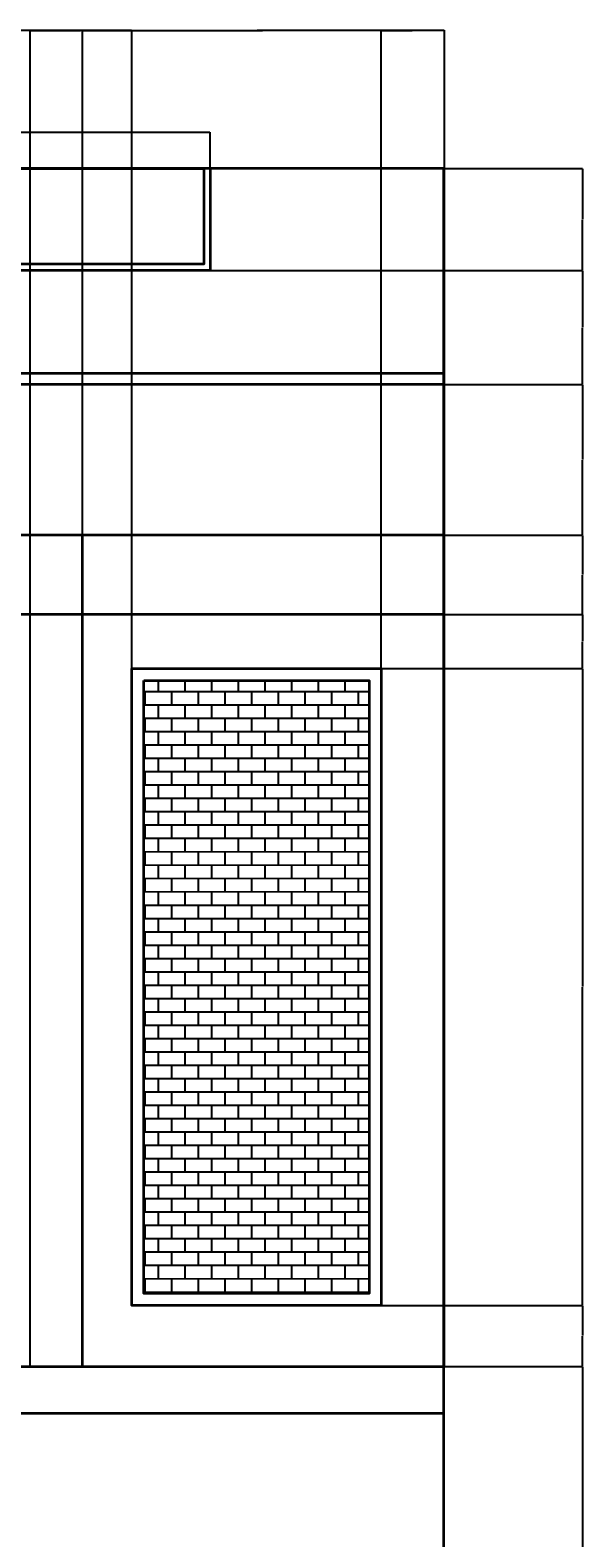
# Model space of a CAD drawing. Units: inches. Extents: x 1231 to 2151, y 481 to 2277.
# Tile 7 of 7: x 1819 to 2151, y 1373 to 2277. Entities that reach past the tile are written whole.
import ezdxf

# ---------------------------------------------------------------- set-up
doc = ezdxf.new("R2010")
doc.units = ezdxf.units.IN
doc.header["$MEASUREMENT"] = 0
for name, color, linetype, lineweight in [('A-ANNO-DIMS', 2, 'Continuous', 18), ('A-ELEV', 7, 'Continuous', 35), ('A-WALL-PATT', 8, 'Continuous', 13)]:
    doc.layers.add(name, color=color, linetype=linetype, lineweight=lineweight)
doc.styles.get("Standard").update_dxf_attribs({"font": 'arial.ttf'})
doc.dimstyles.get("Standard").update_dxf_attribs({"dimtxt": 0.18, "dimasz": 0.18, "dimexe": 0.18, "dimexo": 0.0625, "dimgap": 0.09, "dimtad": 0, "dimtih": 1, "dimtoh": 1, "dimdec": 0, "dimzin": 0, "dimdsep": 46, "dimlunit": 3, "dimtxsty": 'Standard', "dimcen": 0.09, "dimadec": 0, "dimazin": 0, "dimtfac": 1, "dimtdec": 0, "dimtofl": 0, "dimtmove": 0, "dimatfit": 3, "dimfxl": 1, "dimtolj": 1, "dimtzin": 0, "dimarcsym": 0})

# ---------------------------------------------------------------- blocks, each defined once
blk = doc.blocks.new('*D7')
at = {"layer": 'A-ANNO-DIMS', "color": 0, "lineweight": -2, "transparency": 16777216}
for p, q in [((2067.75, 1475.54), (2150.62, 1475.54)), ((2150.44, 1475.36), (2150.44, 1323.12)), ((2150.44, 1170.52), (2150.44, 1322.76)), ((2067.75, 1170.34), (2150.62, 1170.34))]:
    blk.add_line(p, q, dxfattribs=at)
at = {"layer": 'A-ANNO-DIMS', "color": 0, "transparency": 16777216}
for points in [[(2150.41, 1475.36), (2150.47, 1475.36), (2150.44, 1475.54)], [(2150.41, 1170.52), (2150.47, 1170.52), (2150.44, 1170.34)]]:
    blk.add_solid(points, dxfattribs=at)
at = {"layer": 'Defpoints', "color": 0, "transparency": 16777216}
for p in [(2067.69, 1475.54), (2150.44, 1475.54), (2067.69, 1170.34)]:
    blk.add_point(p, dxfattribs=at)
at = {"layer": 'A-ANNO-DIMS', "color": 0, "transparency": 16777216, "insert": (2150.44, 1322.94), "char_height": 0.18, "attachment_point": 5}
blk.add_mtext('\\A1;305.2', dxfattribs=at)
blk = doc.blocks.new('*D8')
at = {"layer": 'A-ANNO-DIMS', "color": 0, "lineweight": -2, "transparency": 16777216}
for p, q in [((2029.92, 1512.17), (2150.62, 1512.17)), ((2150.44, 1511.99), (2150.44, 1494.04)), ((2150.44, 1475.72), (2150.44, 1493.68)), ((2067.75, 1475.54), (2150.62, 1475.54))]:
    blk.add_line(p, q, dxfattribs=at)
at = {"layer": 'A-ANNO-DIMS', "color": 0, "transparency": 16777216}
for points in [[(2150.41, 1511.99), (2150.47, 1511.99), (2150.44, 1512.17)], [(2150.41, 1475.72), (2150.47, 1475.72), (2150.44, 1475.54)]]:
    blk.add_solid(points, dxfattribs=at)
at = {"layer": 'Defpoints', "color": 0, "transparency": 16777216}
for p in [(2029.86, 1512.17), (2150.44, 1512.17), (2067.69, 1475.54)]:
    blk.add_point(p, dxfattribs=at)
at = {"layer": 'A-ANNO-DIMS', "color": 0, "transparency": 16777216, "insert": (2150.44, 1493.86), "char_height": 0.18, "attachment_point": 5}
blk.add_mtext('\\A1;36.63', dxfattribs=at)
blk = doc.blocks.new('*D9')
at = {"layer": 'A-ANNO-DIMS', "color": 0, "lineweight": -2, "transparency": 16777216}
for p, q in [((2029.92, 1894.05), (2150.62, 1894.05)), ((2150.44, 1893.87), (2150.44, 1703.3)), ((2150.44, 1512.35), (2150.44, 1702.93)), ((2029.92, 1512.17), (2150.62, 1512.17))]:
    blk.add_line(p, q, dxfattribs=at)
at = {"layer": 'A-ANNO-DIMS', "color": 0, "transparency": 16777216}
for points in [[(2150.41, 1893.87), (2150.47, 1893.87), (2150.44, 1894.05)], [(2150.41, 1512.35), (2150.47, 1512.35), (2150.44, 1512.17)]]:
    blk.add_solid(points, dxfattribs=at)
at = {"layer": 'Defpoints', "color": 0, "transparency": 16777216}
for p in [(2029.86, 1894.05), (2150.44, 1894.05), (2029.86, 1512.17)]:
    blk.add_point(p, dxfattribs=at)
at = {"layer": 'A-ANNO-DIMS', "color": 0, "transparency": 16777216, "insert": (2150.44, 1703.11), "char_height": 0.18, "attachment_point": 5}
blk.add_mtext('\\A1;381.9', dxfattribs=at)
blk = doc.blocks.new('*D10')
at = {"layer": 'A-ANNO-DIMS', "color": 0, "lineweight": -2, "transparency": 16777216}
for p, q in [((2067.75, 1926.29), (2150.62, 1926.29)), ((2150.44, 1926.11), (2150.44, 1910.35)), ((2150.44, 1894.23), (2150.44, 1909.99)), ((2029.92, 1894.05), (2150.62, 1894.05))]:
    blk.add_line(p, q, dxfattribs=at)
at = {"layer": 'A-ANNO-DIMS', "color": 0, "transparency": 16777216}
for points in [[(2150.41, 1926.11), (2150.47, 1926.11), (2150.44, 1926.29)], [(2150.41, 1894.23), (2150.47, 1894.23), (2150.44, 1894.05)]]:
    blk.add_solid(points, dxfattribs=at)
at = {"layer": 'Defpoints', "color": 0, "transparency": 16777216}
for p in [(2067.69, 1926.29), (2150.44, 1926.29), (2029.86, 1894.05)]:
    blk.add_point(p, dxfattribs=at)
at = {"layer": 'A-ANNO-DIMS', "color": 0, "transparency": 16777216, "insert": (2150.44, 1910.17), "char_height": 0.18, "attachment_point": 5}
blk.add_mtext('\\A1;32.23', dxfattribs=at)
blk = doc.blocks.new('*D11')
at = {"layer": 'A-ANNO-DIMS', "color": 0, "lineweight": -2, "transparency": 16777216}
for p, q in [((2067.75, 1973.89), (2150.62, 1973.89)), ((2150.44, 1973.71), (2150.44, 1950.27)), ((2150.44, 1926.47), (2150.44, 1949.9)), ((2067.75, 1926.29), (2150.62, 1926.29))]:
    blk.add_line(p, q, dxfattribs=at)
at = {"layer": 'A-ANNO-DIMS', "color": 0, "transparency": 16777216}
for points in [[(2150.41, 1973.71), (2150.47, 1973.71), (2150.44, 1973.89)], [(2150.41, 1926.47), (2150.47, 1926.47), (2150.44, 1926.29)]]:
    blk.add_solid(points, dxfattribs=at)
at = {"layer": 'Defpoints', "color": 0, "transparency": 16777216}
for p in [(2067.69, 1973.89), (2150.44, 1973.89), (2067.69, 1926.29)]:
    blk.add_point(p, dxfattribs=at)
at = {"layer": 'A-ANNO-DIMS', "color": 0, "transparency": 16777216, "insert": (2150.44, 1950.09), "char_height": 0.18, "attachment_point": 5}
blk.add_mtext('\\A1;47.6', dxfattribs=at)
blk = doc.blocks.new('*D12')
at = {"layer": 'A-ANNO-DIMS', "color": 0, "lineweight": -2, "transparency": 16777216}
for p, q in [((2067.75, 2064.21), (2150.62, 2064.21)), ((2150.44, 2064.03), (2150.44, 2019.23)), ((2150.44, 1974.07), (2150.44, 2018.87)), ((2067.75, 1973.89), (2150.62, 1973.89))]:
    blk.add_line(p, q, dxfattribs=at)
at = {"layer": 'A-ANNO-DIMS', "color": 0, "transparency": 16777216}
for points in [[(2150.41, 2064.03), (2150.47, 2064.03), (2150.44, 2064.21)], [(2150.41, 1974.07), (2150.47, 1974.07), (2150.44, 1973.89)]]:
    blk.add_solid(points, dxfattribs=at)
at = {"layer": 'Defpoints', "color": 0, "transparency": 16777216}
for p in [(2067.69, 2064.21), (2150.44, 2064.21), (2067.69, 1973.89)]:
    blk.add_point(p, dxfattribs=at)
at = {"layer": 'A-ANNO-DIMS', "color": 0, "transparency": 16777216, "insert": (2150.44, 2019.05), "char_height": 0.18, "attachment_point": 5}
blk.add_mtext('\\A1;90.33', dxfattribs=at)
blk = doc.blocks.new('*D13')
at = {"layer": 'A-ANNO-DIMS', "color": 0, "lineweight": -2, "transparency": 16777216}
for p, q in [((1927.34, 2132.55), (2150.62, 2132.55)), ((2150.44, 2132.37), (2150.44, 2098.56)), ((2150.44, 2064.39), (2150.44, 2098.2)), ((2067.75, 2064.21), (2150.62, 2064.21))]:
    blk.add_line(p, q, dxfattribs=at)
at = {"layer": 'A-ANNO-DIMS', "color": 0, "transparency": 16777216}
for points in [[(2150.41, 2132.37), (2150.47, 2132.37), (2150.44, 2132.55)], [(2150.41, 2064.39), (2150.47, 2064.39), (2150.44, 2064.21)]]:
    blk.add_solid(points, dxfattribs=at)
at = {"layer": 'Defpoints', "color": 0, "transparency": 16777216}
for p in [(1927.28, 2132.55), (2150.44, 2132.55), (2067.69, 2064.21)]:
    blk.add_point(p, dxfattribs=at)
at = {"layer": 'A-ANNO-DIMS', "color": 0, "transparency": 16777216, "insert": (2150.44, 2098.38), "char_height": 0.18, "attachment_point": 5}
blk.add_mtext('\\A1;68.34', dxfattribs=at)
blk = doc.blocks.new('*D14')
at = {"layer": 'A-ANNO-DIMS', "color": 0, "lineweight": -2, "transparency": 16777216}
for p, q in [((2067.54, 2193.78), (2150.62, 2193.78)), ((2150.44, 2193.6), (2150.44, 2163.35)), ((2150.44, 2132.73), (2150.44, 2162.98)), ((1927.34, 2132.55), (2150.62, 2132.55))]:
    blk.add_line(p, q, dxfattribs=at)
at = {"layer": 'A-ANNO-DIMS', "color": 0, "transparency": 16777216}
for points in [[(2150.41, 2193.6), (2150.47, 2193.6), (2150.44, 2193.78)], [(2150.41, 2132.73), (2150.47, 2132.73), (2150.44, 2132.55)]]:
    blk.add_solid(points, dxfattribs=at)
at = {"layer": 'Defpoints', "color": 0, "transparency": 16777216}
for p in [(2067.47, 2193.78), (2150.44, 2193.78), (1927.28, 2132.55)]:
    blk.add_point(p, dxfattribs=at)
at = {"layer": 'A-ANNO-DIMS', "color": 0, "transparency": 16777216, "insert": (2150.44, 2163.16), "char_height": 0.18, "attachment_point": 5}
blk.add_mtext('\\A1;61.23', dxfattribs=at)
blk = doc.blocks.new('*D18')
at = {"layer": 'A-ANNO-DIMS', "color": 0, "lineweight": -2, "transparency": 16777216}
for p, q in [((1562.79, 1914.62), (1562.79, 2276.71)), ((1562.97, 2276.53), (1690.65, 2276.53)), ((1819.13, 2276.53), (1691.45, 2276.53)), ((1819.31, 1914.62), (1819.31, 2276.71))]:
    blk.add_line(p, q, dxfattribs=at)
at = {"layer": 'A-ANNO-DIMS', "color": 0, "transparency": 16777216}
for points in [[(1562.97, 2276.56), (1562.97, 2276.5), (1562.79, 2276.53)], [(1819.13, 2276.56), (1819.13, 2276.5), (1819.31, 2276.53)]]:
    blk.add_solid(points, dxfattribs=at)
at = {"layer": 'Defpoints', "color": 0, "transparency": 16777216}
for p in [(1819.31, 2276.53), (1562.79, 1914.56), (1819.31, 1914.56)]:
    blk.add_point(p, dxfattribs=at)
at = {"layer": 'A-ANNO-DIMS', "color": 0, "transparency": 16777216, "insert": (1691.05, 2276.53), "char_height": 0.18, "attachment_point": 5}
blk.add_mtext('\\A1;256.5', dxfattribs=at)
blk = doc.blocks.new('*D19')
at = {"layer": 'A-ANNO-DIMS', "color": 0, "lineweight": -2, "transparency": 16777216}
for p, q in [((1819.31, 1475.61), (1819.31, 2276.71)), ((1819.49, 2276.53), (1849.41, 2276.53)), ((1880.11, 2276.53), (1850.19, 2276.53)), ((1880.29, 1512.24), (1880.29, 2276.71))]:
    blk.add_line(p, q, dxfattribs=at)
at = {"layer": 'A-ANNO-DIMS', "color": 0, "transparency": 16777216}
for points in [[(1819.49, 2276.56), (1819.49, 2276.5), (1819.31, 2276.53)], [(1880.11, 2276.56), (1880.11, 2276.5), (1880.29, 2276.53)]]:
    blk.add_solid(points, dxfattribs=at)
at = {"layer": 'Defpoints', "color": 0, "transparency": 16777216}
for p in [(1880.29, 2276.53), (1880.29, 1512.17), (1819.31, 1475.54)]:
    blk.add_point(p, dxfattribs=at)
at = {"layer": 'A-ANNO-DIMS', "color": 0, "transparency": 16777216, "insert": (1849.8, 2276.53), "char_height": 0.18, "attachment_point": 5}
blk.add_mtext('\\A1;60.98', dxfattribs=at)
blk = doc.blocks.new('*D20')
at = {"layer": 'A-ANNO-DIMS', "color": 0, "lineweight": -2, "transparency": 16777216}
for p, q in [((1880.29, 1512.24), (1880.29, 2276.71)), ((1880.47, 2276.53), (1954.62, 2276.53)), ((2029.68, 2276.53), (1955.53, 2276.53)), ((2029.86, 1512.24), (2029.86, 2276.71))]:
    blk.add_line(p, q, dxfattribs=at)
at = {"layer": 'A-ANNO-DIMS', "color": 0, "transparency": 16777216}
for points in [[(1880.47, 2276.56), (1880.47, 2276.5), (1880.29, 2276.53)], [(2029.68, 2276.56), (2029.68, 2276.5), (2029.86, 2276.53)]]:
    blk.add_solid(points, dxfattribs=at)
at = {"layer": 'Defpoints', "color": 0, "transparency": 16777216}
for p in [(2029.86, 2276.53), (1880.29, 1512.17), (2029.86, 1512.17)]:
    blk.add_point(p, dxfattribs=at)
at = {"layer": 'A-ANNO-DIMS', "color": 0, "transparency": 16777216, "insert": (1955.08, 2276.53), "char_height": 0.18, "attachment_point": 5}
blk.add_mtext('\\A1;149.57', dxfattribs=at)
blk = doc.blocks.new('*D21')
at = {"layer": 'A-ANNO-DIMS', "color": 0, "lineweight": -2, "transparency": 16777216}
for p, q in [((2029.86, 1512.24), (2029.86, 2276.71)), ((2030.04, 2276.53), (2048.38, 2276.53)), ((2067.51, 2276.53), (2049.17, 2276.53)), ((2067.69, 1475.61), (2067.69, 2276.71))]:
    blk.add_line(p, q, dxfattribs=at)
at = {"layer": 'A-ANNO-DIMS', "color": 0, "transparency": 16777216}
for points in [[(2030.04, 2276.56), (2030.04, 2276.5), (2029.86, 2276.53)], [(2067.51, 2276.56), (2067.51, 2276.5), (2067.69, 2276.53)]]:
    blk.add_solid(points, dxfattribs=at)
at = {"layer": 'Defpoints', "color": 0, "transparency": 16777216}
for p in [(2067.69, 2276.53), (2029.86, 1512.17), (2067.69, 1475.54)]:
    blk.add_point(p, dxfattribs=at)
at = {"layer": 'A-ANNO-DIMS', "color": 0, "transparency": 16777216, "insert": (2048.77, 2276.53), "char_height": 0.18, "attachment_point": 5}
blk.add_mtext('\\A1;37.83', dxfattribs=at)
blk = doc.blocks.new('*D23')
at = {"layer": 'A-ANNO-DIMS', "color": 0, "lineweight": -2, "transparency": 16777216}
for p, q in [((1531.21, 1973.95), (1531.21, 2276.71)), ((1531.39, 2276.53), (1690.57, 2276.53)), ((1850.54, 2276.53), (1691.36, 2276.53)), ((1850.72, 1973.95), (1850.72, 2276.71))]:
    blk.add_line(p, q, dxfattribs=at)
at = {"layer": 'A-ANNO-DIMS', "color": 0, "transparency": 16777216}
for points in [[(1531.39, 2276.56), (1531.39, 2276.5), (1531.21, 2276.53)], [(1850.54, 2276.56), (1850.54, 2276.5), (1850.72, 2276.53)]]:
    blk.add_solid(points, dxfattribs=at)
at = {"layer": 'Defpoints', "color": 0, "transparency": 16777216}
for p in [(1850.72, 2276.53), (1531.21, 1973.89), (1850.72, 1973.89)]:
    blk.add_point(p, dxfattribs=at)
at = {"layer": 'A-ANNO-DIMS', "color": 0, "transparency": 16777216, "insert": (1690.96, 2276.53), "char_height": 0.18, "attachment_point": 5}
blk.add_mtext('\\A1;319.5', dxfattribs=at)
blk = doc.blocks.new('*D24')
at = {"layer": 'A-ANNO-DIMS', "color": 0, "lineweight": -2, "transparency": 16777216}
for p, q in [((1850.72, 1973.95), (1850.72, 2276.71)), ((1850.9, 2276.53), (1958.74, 2276.53)), ((2067.51, 2276.53), (1959.67, 2276.53)), ((2067.69, 1973.95), (2067.69, 2276.71))]:
    blk.add_line(p, q, dxfattribs=at)
at = {"layer": 'A-ANNO-DIMS', "color": 0, "transparency": 16777216}
for points in [[(1850.9, 2276.56), (1850.9, 2276.5), (1850.72, 2276.53)], [(2067.51, 2276.56), (2067.51, 2276.5), (2067.69, 2276.53)]]:
    blk.add_solid(points, dxfattribs=at)
at = {"layer": 'Defpoints', "color": 0, "transparency": 16777216}
for p in [(2067.69, 2276.53), (1850.72, 1973.89), (2067.69, 1973.89)]:
    blk.add_point(p, dxfattribs=at)
at = {"layer": 'A-ANNO-DIMS', "color": 0, "transparency": 16777216, "insert": (1959.2, 2276.53), "char_height": 0.18, "attachment_point": 5}
blk.add_mtext('\\A1;216.97', dxfattribs=at)
blk = doc.blocks.new('*D26')
at = {"layer": 'A-ANNO-DIMS', "color": 0, "lineweight": -2, "transparency": 16777216}
for p, q in [((1509.79, 2132.61), (1509.79, 2215.48)), ((1509.97, 2215.3), (1718.14, 2215.3)), ((1927.1, 2215.3), (1718.93, 2215.3)), ((1927.28, 2132.61), (1927.28, 2215.48))]:
    blk.add_line(p, q, dxfattribs=at)
at = {"layer": 'A-ANNO-DIMS', "color": 0, "transparency": 16777216}
for points in [[(1509.97, 2215.33), (1509.97, 2215.27), (1509.79, 2215.3)], [(1927.1, 2215.33), (1927.1, 2215.27), (1927.28, 2215.3)]]:
    blk.add_solid(points, dxfattribs=at)
at = {"layer": 'Defpoints', "color": 0, "transparency": 16777216}
for p in [(1927.28, 2215.3), (1509.79, 2132.55), (1927.28, 2132.55)]:
    blk.add_point(p, dxfattribs=at)
at = {"layer": 'A-ANNO-DIMS', "color": 0, "transparency": 16777216, "insert": (1718.53, 2215.3), "char_height": 0.18, "attachment_point": 5}
blk.add_mtext('\\A1;417.5', dxfattribs=at)

msp = doc.modelspace()

# ---------------------------------------------------------------- hatches: boundary and pattern name
at = {"layer": 'A-WALL-PATT'}
h = msp.add_hatch(dxfattribs=at)
h.set_pattern_fill('AR-B816C', color=256)
h.set_pattern_definition([(0, (536.475, 2e-13), (8, 8), [15.625, -0.375]), (0, (528.475, 0.375), (8, 8), [15.625, -0.375]), (90, (536.475, 2e-13), (-8, 8), [-8.375, 7.625]), (90, (536.1, 2e-13), (-8, 8), [-8.375, 7.625])])
h.paths.add_polyline_path([(2022.6824, 1886.877), (1887.4677, 1886.877), (1887.4677, 1519.3518), (2022.6824, 1519.3518)])

# ---------------------------------------------------------------- linework, layer by layer
at = {"layer": 'A-ELEV'}
for p, q in [((2067.6855, 2193.7789), (1314.2408, 2193.7789)), ((2067.4747, 563.6912), (2067.4747, 2193.7789)), ((2067.6855, 2070.8244), (1314.2408, 2070.8244)), ((2067.6855, 2064.2116), (1314.2408, 2064.2116)), ((2067.6855, 1973.8854), (1314.2408, 1973.8854)), ((1850.716, 1475.5441), (1850.716, 1973.8854)), ((2067.6855, 1926.2862), (1314.2408, 1926.2862)), ((1314.2408, 1475.5441), (2067.6855, 1475.5441)), ((1498.3132, 1447.5396), (2067.6855, 1447.5396))]:
    msp.add_line(p, q, dxfattribs=at)
msp.add_lwpolyline([(1927.277, 2193.7789), (1927.277, 2132.5472), (1509.7902, 2132.5472), (1509.7902, 2193.7789)], dxfattribs=at)
for points in [[(1513.6622, 2193.7789), (1923.405, 2193.7789), (1923.405, 2136.4192), (1513.6622, 2136.4192)], [(1880.2909, 1894.0538), (2029.8592, 1894.0538), (2029.8592, 1512.1749), (1880.2909, 1512.1749)], [(1887.4677, 1886.877), (2022.6824, 1886.877), (2022.6824, 1519.3518), (1887.4677, 1519.3518)]]:
    msp.add_lwpolyline(points, close=True, dxfattribs=at)

# ---------------------------------------------------------------- dimensions: what is measured, and where the dimension line sits
at = {"layer": 'A-ANNO-DIMS'}
for base, p1, p2, override, picture, middle in [((1850.716, 2276.5289), (1531.2103, 1973.8854), (1850.716, 1973.8854), {"dimdec": 1, "dimlfac": 1, "dimrnd": 0, "dimzin": 0, "dimdsep": 46, "dimlunit": 2}, '*D23', (1690.9632, 2276.5289)), ((1819.3087, 2276.5289), (1562.7916, 1914.557), (1819.3087, 1914.557), {"dimdec": 1, "dimlfac": 1, "dimrnd": 0, "dimzin": 0, "dimdsep": 46, "dimlunit": 2}, '*D18', (1691.0501, 2276.5289)), ((1880.2909, 2276.5289), (1819.3087, 1475.5441), (1880.2909, 1512.1749), {"dimdec": 2, "dimlfac": 1, "dimrnd": 0, "dimzin": 0, "dimdsep": 46, "dimlunit": 2}, '*D19', (1849.7998, 2276.5289)), ((2067.6855, 2276.5289), (1850.716, 1973.8854), (2067.6855, 1973.8854), {"dimdec": 2, "dimlfac": 1, "dimrnd": 0, "dimzin": 0, "dimdsep": 46, "dimlunit": 2}, '*D24', (1959.2007, 2276.5289)), ((2029.8592, 2276.5289), (1880.2909, 1512.1749), (2029.8592, 1512.1749), {"dimdec": 2, "dimlfac": 1, "dimrnd": 0, "dimzin": 0, "dimdsep": 46, "dimlunit": 2}, '*D20', (1955.0751, 2276.5289)), ((2067.6855, 2276.5289), (2029.8592, 1512.1749), (2067.6855, 1475.5441), {"dimdec": 2, "dimlfac": 1, "dimrnd": 0, "dimzin": 0, "dimdsep": 46, "dimlunit": 2}, '*D21', (2048.7724, 2276.5289)), ((1927.277, 2215.2972), (1509.7902, 2132.5472), (1927.277, 2132.5472), {"dimdec": 1, "dimlfac": 1, "dimrnd": 0, "dimzin": 0, "dimdsep": 46, "dimlunit": 2}, '*D26', (1718.5336, 2215.2972))]:
    dim = msp.add_linear_dim(base=base, p1=p1, p2=p2, dimstyle='Standard', override=override, dxfattribs=at)
    dim.commit()
    dim.dimension.update_dxf_attribs({"geometry": picture, "text_midpoint": middle})
for base, p1, p2, override, picture, middle in [((2150.4355, 2193.7789), (1927.277, 2132.5472), (2067.4747, 2193.7789), {"dimdec": 2, "dimlfac": 1, "dimrnd": 0, "dimzin": 0, "dimdsep": 46, "dimlunit": 2}, '*D14', (2150.4355, 2163.1631)), ((2150.4355, 2132.5472), (2067.6855, 2064.2116), (1927.277, 2132.5472), {"dimdec": 2, "dimlfac": 1, "dimrnd": 0, "dimzin": 0, "dimdsep": 46, "dimlunit": 2}, '*D13', (2150.4355, 2098.3794)), ((2150.4355, 2064.2116), (2067.6855, 1973.8854), (2067.6855, 2064.2116), {"dimdec": 2, "dimlfac": 1, "dimrnd": 0, "dimzin": 0, "dimdsep": 46, "dimlunit": 2}, '*D12', (2150.4355, 2019.0485)), ((2150.4355, 1973.8854), (2067.6855, 1926.2862), (2067.6855, 1973.8854), {"dimdec": 1, "dimlfac": 1, "dimrnd": 0, "dimzin": 0, "dimdsep": 46, "dimlunit": 2}, '*D11', (2150.4355, 1950.0858)), ((2150.4355, 1926.2862), (2029.8592, 1894.0538), (2067.6855, 1926.2862), {"dimdec": 2, "dimlfac": 1, "dimrnd": 0, "dimzin": 0, "dimdsep": 46, "dimlunit": 2}, '*D10', (2150.4355, 1910.17)), ((2150.4355, 1894.0538), (2029.8592, 1512.1749), (2029.8592, 1894.0538), {"dimdec": 1, "dimlfac": 1, "dimrnd": 0, "dimzin": 0, "dimdsep": 46, "dimlunit": 2}, '*D9', (2150.4355, 1703.1144)), ((2150.4355, 1512.1749), (2067.6855, 1475.5441), (2029.8592, 1512.1749), {"dimdec": 2, "dimlfac": 1, "dimrnd": 0, "dimzin": 0, "dimdsep": 46, "dimlunit": 2}, '*D8', (2150.4355, 1493.8595)), ((2150.4355, 1475.5441), (2067.6855, 1170.3352), (2067.6855, 1475.5441), {"dimdec": 1, "dimlfac": 1, "dimrnd": 0, "dimzin": 0, "dimdsep": 46, "dimlunit": 2}, '*D7', (2150.4355, 1322.9396))]:
    dim = msp.add_linear_dim(base=base, p1=p1, p2=p2, angle=90, dimstyle='Standard', override=override, dxfattribs=at)
    dim.commit()
    dim.dimension.update_dxf_attribs({"geometry": picture, "text_midpoint": middle})

doc.saveas('drawing.dxf')
